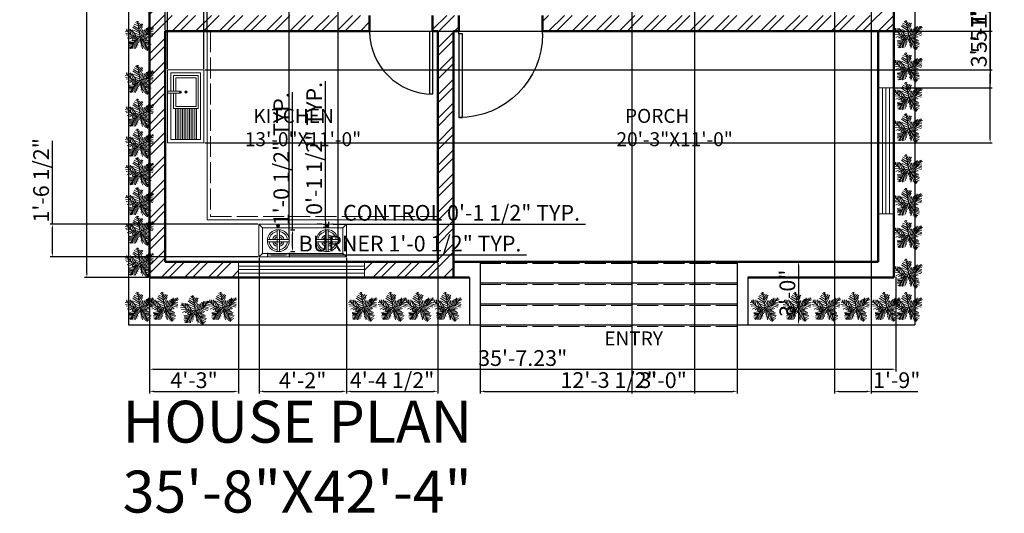
# Model space of a CAD drawing. Units: inches. Extents: x 176 to 806, y 915 to 1663.
# Tile 1 of 5: x 228 to 792, y 915 to 1198. Entities that reach past the tile are written whole.
import ezdxf

# ---------------------------------------------------------------- set-up
doc = ezdxf.new("R2010")
doc.units = ezdxf.units.IN
doc.linetypes.add('ACAD_ISO02W100', pattern=[15, 12, -3])
for name, color, linetype, lineweight in [('A-ANNO-DIMS', 2, 'Continuous', 18), ('A-ANNO-TEXT', 7, 'Continuous', 18), ('A-AREA-IDEN', 7, 'Continuous', 18), ('A-DOOR', 4, 'Continuous', 25), ('A-EQPM', 9, 'Continuous', 18), ('A-FLOR-CASE', 8, 'Continuous', 18), ('A-FLOR-CASE-HIDN', 8, 'ACAD_ISO02W100', 13), ('A-FLOR-FIXT', 9, 'Continuous', 18), ('A-FLOR-STRS', 7, 'Continuous', 25), ('A-FLOR-STRS-HIDN', 8, 'ACAD_ISO02W100', 13), ('A-WALL', 7, 'Continuous', 50), ('A-WALL-PATT', 252, 'Continuous', 13), ('C-PROP', 8, 'Continuous', 25), ('L-PLNT', 3, 'Continuous', 13)]:
    doc.layers.add(name, color=color, linetype=linetype, lineweight=lineweight)
doc.layers.add('A-GLAZ', color=244, linetype='Continuous', lineweight=18, true_color=0x991b1e)
doc.styles.get("Standard").update_dxf_attribs({"font": 'arial.ttf'})
doc.dimstyles.new('ISO-25', dxfattribs={"dimtxt": 9, "dimasz": 2.5, "dimexe": 1.25, "dimexo": 0.625, "dimtad": 1, "dimlunit": 3, "dimtxsty": 'Standard', "dimcen": 2.5, "dimadec": 0, "dimazin": 0, "dimtfac": 1, "dimtmove": 0, "dimatfit": 3, "dimfxl": 1, "dimarcsym": 0})

# ---------------------------------------------------------------- blocks, each defined once
blk = doc.blocks.new('*U2')
for p, q in [((-40, 0), (-40, 6)), ((0, 0), (0, 6))]:
    blk.add_line(p, q)
blk.add_lwpolyline([(0, 0), (0, -40), (-1.75, -40), (-1.75, 0)], close=True)
blk.add_arc((0, 0), 40, 180, 270)
blk = doc.blocks.new('*U8')
for p, q in [((-5.114, 28.097), (-24.676, 40.636)), ((-7.288, 39.707), (-21.778, 46.673)), ((-8.737, 47.138), (-17.069, 52.711)), ((-10.186, 53.64), (-13.084, 55.962)), ((0, 0), (-10.5, 57)), ((-9.099, 51.782), (-6.563, 55.962)), ((-7.65, 43.423), (-2.578, 49.46)), ((-5.839, 35.992), (4.667, 48.067)), ((-5.114, 27.632), (10.463, 46.673)), ((-2.941, 16.486), (8.652, 37.85)), ((-47.498, 19.737), (-55.83, 18.344)), ((-40.615, 13.7), (-55.105, 10.913)), ((-31.5, 4.5), (-52.5, 25.5)), ((-33.37, 6.269), (-52.207, 5.34)), ((-48.585, 21.131), (-49.309, 29.026)), ((-28.299, 3.483), (-47.86, -5.805)), ((-43.513, 28.561), (-42.427, 15.558)), ((-38.442, 26.239), (-34.819, 7.663)), ((-21.416, 3.018), (-38.079, -8.128)), ((-35.544, 28.097), (-24.314, 3.947)), ((0, 0), (-31.5, 4.5)), ((-14.533, 2.09), (-30.834, 25.31)), ((-15.982, 2.09), (-30.11, -9.521)), ((-3.665, 19.273), (-27.574, 35.527)), ((-24.314, 23.917), (-2.941, 13.7)), ((0, 0), (-22.5, -19.5)), ((-6.563, 1.161), (-21.416, -8.128)), ((-20.691, 13.7), (-1.129, 4.876)), ((-1.129, 6.734), (9.014, 26.704)), ((0, 0), (27, 9)), ((0, 0), (18, -22.5)), ((3.942, 1.625), (11.187, 24.381)), ((6.478, 1.625), (26.04, -8.592)), ((10.101, 3.483), (17.708, 26.239)), ((11.187, 3.483), (30.749, -5.805)), ((16.259, 5.805), (23.142, 31.348)), ((18.07, 5.805), (35.096, -3.483)), ((22.055, 7.198), (27.489, 32.277)), ((24.229, 7.663), (46.688, 1.625)), ((27, 9), (48, 36)), ((27.127, 9.056), (31.112, 35.992)), ((29.662, 12.307), (48.137, 6.269)), ((31.836, 30.883), (32.561, 16.486)), ((33.285, 16.486), (48.862, 10.913)), ((35.096, 32.741), (37.27, 22.524)), ((36.183, 19.737), (48.137, 17.88)), ((38.719, 34.134), (41.979, 28.561)), ((40.53, 25.775), (48.862, 24.846)), ((43.791, 29.954), (51.036, 30.883)), ((44.153, 36.456), (45.239, 32.741)), ((-17.431, -15.094), (-42.789, -18.809)), ((-28.299, -29.026), (-42.789, -31.348)), ((-24.314, -21.596), (-42.427, -22.06)), ((-30.834, -34.135), (-42.427, -35.528)), ((-26.849, -26.24), (-40.253, -25.775)), ((-22.5, -19.5), (-37.5, -45)), ((-15.257, -12.772), (-30.11, -12.772)), ((-29.023, -30.884), (-27.936, -43.887)), ((-25.038, -23.918), (-22.865, -45.281)), ((-20.691, -18.345), (-17.793, -44.352)), ((-6.563, -5.805), (-19.967, -9.985)), ((-17.069, -15.094), (-12.721, -40.172)), ((-13.446, -11.378), (-8.737, -32.741)), ((-9.461, -8.592), (-6.201, -23.453)), ((-4.752, -3.483), (-3.665, -14.629)), ((2.493, -3.019), (-1.491, -20.202)), ((1.769, -2.555), (24.229, -9.521)), ((5.029, -6.27), (2.131, -25.775)), ((9.014, -11.378), (3.58, -35.992)), ((14.085, -16.951), (6.478, -40.172)), ((7.565, -9.056), (32.198, -14.629)), ((18.07, -22.524), (8.289, -45.745)), ((12.274, -15.094), (36.907, -18.809)), ((20.244, -30.419), (15.897, -44.816)), ((16.259, -19.738), (36.183, -22.989)), ((18, -22.5), (27, -52.5)), ((18.433, -22.524), (40.53, -29.026)), ((19.157, -25.311), (38.719, -33.206)), ((21.331, -32.741), (39.081, -40.636)), ((-34.457, -39.708), (-40.978, -42.494)), ((-32.646, -36.921), (-31.921, -44.352)), ((22.78, -37.85), (19.519, -48.532)), ((22.78, -38.314), (34.372, -44.816)), ((24.591, -45.745), (23.142, -50.854)), ((24.591, -43.423), (30.749, -47.603)), ((26.764, -49.925), (28.213, -50.854))]:
    blk.add_line(p, q)
blk = doc.blocks.new('*D9')
at = {"layer": 'A-ANNO-DIMS', "color": 0, "lineweight": -2, "transparency": 16777216}
for p, q in [((302.7, 1049.58), (302.7, 996.47)), ((729.94, 1050.58), (729.94, 996.47)), ((305.2, 997.72), (727.44, 997.72))]:
    blk.add_line(p, q, dxfattribs=at)
at = {"layer": 'A-ANNO-DIMS', "color": 0, "transparency": 16777216}
for points in [[(305.2, 998.13), (305.2, 997.3), (302.7, 997.72)], [(727.44, 998.13), (727.44, 997.3), (729.94, 997.72)]]:
    blk.add_solid(points, dxfattribs=at)
at = {"layer": 'Defpoints', "color": 0, "transparency": 16777216}
for p in [(302.7, 1050.21), (729.94, 1051.2), (729.94, 997.72)]:
    blk.add_point(p, dxfattribs=at)
at = {"layer": 'A-ANNO-DIMS', "color": 0, "transparency": 16777216, "insert": (516.32, 1002.94), "char_height": 9, "attachment_point": 5}
blk.add_mtext('35\'-7.23"', dxfattribs=at)
blk = doc.blocks.new('*D10')
at = {"layer": 'A-ANNO-DIMS', "color": 0, "lineweight": -2, "transparency": 16777216}
for p, q in [((302.08, 1558.21), (265.58, 1558.21)), ((266.83, 1052.71), (266.83, 1555.71)), ((302.08, 1050.21), (265.58, 1050.21))]:
    blk.add_line(p, q, dxfattribs=at)
at = {"layer": 'A-ANNO-DIMS', "color": 0, "transparency": 16777216}
for points in [[(266.42, 1555.71), (267.25, 1555.71), (266.83, 1558.21)], [(266.42, 1052.71), (267.25, 1052.71), (266.83, 1050.21)]]:
    blk.add_solid(points, dxfattribs=at)
at = {"layer": 'Defpoints', "color": 0, "transparency": 16777216}
for p in [(266.83, 1558.21), (302.7, 1558.21), (302.7, 1050.21)]:
    blk.add_point(p, dxfattribs=at)
at = {"layer": 'A-ANNO-DIMS', "color": 0, "transparency": 16777216, "insert": (261.69, 1304.21), "char_height": 9, "attachment_point": 5, "rotation": 90}
blk.add_mtext('42\'-4"', dxfattribs=at)
blk = doc.blocks.new('WIN-GLAZING-72IN')
for p, q in [((0, 2), (72, 2)), ((0, 0), (72, 0)), ((0, -2), (72, -2))]:
    blk.add_line(p, q)
blk = doc.blocks.new('COOKTOP-BURNER')
for p, q in [((-0.6, 6.24), (-0.6, -6.24)), ((0.6, 6.24), (0.6, -6.24)), ((-6.24, 0.6), (6.24, 0.6)), ((-6.24, -0.6), (6.24, -0.6))]:
    blk.add_line(p, q)
blk.add_circle((0, 0), 6.27)
for radius, start, end in [(5.27, 96.5353, 173.4647), (3.27, 100.5674, 169.4326), (2.27, 105.3147, 164.6853), (5.27, 6.5353, 83.4647), (3.27, 10.5674, 79.4326), (2.27, 15.3147, 74.6853), (5.27, 186.5353, 263.4647), (3.27, 190.5674, 259.4326), (2.27, 195.3147, 254.6853), (5.27, 276.5353, 353.4647), (3.27, 280.5674, 349.4326), (2.27, 285.3147, 344.6853)]:
    blk.add_arc((0, 0), radius, start, end)
blk = doc.blocks.new('COOKTOP-CONTROL')
for p, q in [((-0.82, 0.2), (0.82, 0.2)), ((-0.82, -0.2), (0.82, -0.2))]:
    blk.add_line(p, q)
blk.add_circle((0, 0), 0.845)
for start, end in [(21.5247, 158.4753), (201.5247, 338.4753)]:
    blk.add_arc((0, 0), 0.545, start, end)
blk = doc.blocks.new('*D30')
at = {"layer": 'A-ANNO-DIMS', "color": 0, "lineweight": -2, "transparency": 16777216}
for p, q in [((370.15, 1064.42), (370.15, 1061.91)), ((372.65, 1063.16), (380.19, 1063.16)), ((382.69, 1064.42), (382.69, 1061.91)), ((382.69, 1063.16), (518.46, 1063.16))]:
    blk.add_line(p, q, dxfattribs=at)
at = {"layer": 'A-ANNO-DIMS', "color": 0, "transparency": 16777216}
for points in [[(372.65, 1063.58), (372.65, 1062.75), (370.15, 1063.16)], [(380.19, 1063.58), (380.19, 1062.75), (382.69, 1063.16)]]:
    blk.add_solid(points, dxfattribs=at)
at = {"layer": 'Defpoints', "color": 0, "transparency": 16777216}
for p in [(370.15, 1065.04), (382.69, 1065.04), (382.69, 1063.16)]:
    blk.add_point(p, dxfattribs=at)
at = {"layer": 'A-ANNO-DIMS', "color": 0, "transparency": 16777216, "insert": (451.83, 1068.44), "char_height": 9, "attachment_point": 5}
blk.add_mtext('BURNER 1\'-0 1/2" TYP.', dxfattribs=at)
blk = doc.blocks.new('*D31')
at = {"layer": 'A-ANNO-DIMS', "color": 0, "lineweight": -2, "transparency": 16777216}
for p, q in [((384.58, 1077.59), (384.58, 1156.32)), ((383.32, 1077.59), (385.83, 1077.59)), ((384.58, 1067.54), (384.58, 1075.09)), ((383.32, 1065.04), (385.83, 1065.04))]:
    blk.add_line(p, q, dxfattribs=at)
at = {"layer": 'A-ANNO-DIMS', "color": 0, "transparency": 16777216}
for points in [[(384.16, 1075.09), (384.99, 1075.09), (384.58, 1077.59)], [(384.16, 1067.54), (384.99, 1067.54), (384.58, 1065.04)]]:
    blk.add_solid(points, dxfattribs=at)
at = {"layer": 'Defpoints', "color": 0, "transparency": 16777216}
for p in [(382.69, 1077.59), (384.58, 1077.59), (382.69, 1065.04)]:
    blk.add_point(p, dxfattribs=at)
at = {"layer": 'A-ANNO-DIMS', "color": 0, "transparency": 16777216, "insert": (379.3, 1118.2), "char_height": 9, "attachment_point": 5, "rotation": 90}
blk.add_mtext('1\'-0 1/2" TYP.', dxfattribs=at)
blk = doc.blocks.new('*D32')
at = {"layer": 'A-ANNO-DIMS', "color": 0, "lineweight": -2, "transparency": 16777216}
for p, q in [((401.15, 1080.8), (398.65, 1080.8)), ((403.65, 1081.17), (403.65, 1082.05)), ((403.65, 1080.8), (405.34, 1080.8)), ((405.34, 1081.17), (405.34, 1082.05)), ((407.84, 1080.8), (552.28, 1080.8))]:
    blk.add_line(p, q, dxfattribs=at)
at = {"layer": 'A-ANNO-DIMS', "color": 0, "transparency": 16777216}
for points in [[(401.15, 1081.22), (401.15, 1080.38), (403.65, 1080.8)], [(407.84, 1081.22), (407.84, 1080.38), (405.34, 1080.8)]]:
    blk.add_solid(points, dxfattribs=at)
at = {"layer": 'Defpoints', "color": 0, "transparency": 16777216}
for p in [(403.65, 1080.55), (405.34, 1080.8), (405.34, 1080.55)]:
    blk.add_point(p, dxfattribs=at)
at = {"layer": 'A-ANNO-DIMS', "color": 0, "transparency": 16777216, "insert": (481.31, 1086.08), "char_height": 9, "attachment_point": 5}
blk.add_mtext('CONTROL 0\'-1 1/2" TYP.', dxfattribs=at)
blk = doc.blocks.new('*D33')
at = {"layer": 'A-ANNO-DIMS', "color": 0, "lineweight": -2, "transparency": 16777216}
for p, q in [((403.4, 1083.05), (403.4, 1162.63)), ((403.03, 1080.55), (402.15, 1080.55)), ((403.03, 1078.86), (402.15, 1078.86)), ((403.4, 1078.86), (403.4, 1080.55)), ((403.4, 1076.36), (403.4, 1073.86))]:
    blk.add_line(p, q, dxfattribs=at)
at = {"layer": 'A-ANNO-DIMS', "color": 0, "transparency": 16777216}
for points in [[(402.98, 1083.05), (403.81, 1083.05), (403.4, 1080.55)], [(402.98, 1076.36), (403.81, 1076.36), (403.4, 1078.86)]]:
    blk.add_solid(points, dxfattribs=at)
at = {"layer": 'Defpoints', "color": 0, "transparency": 16777216}
for p in [(403.4, 1080.55), (403.65, 1080.55), (403.65, 1078.86)]:
    blk.add_point(p, dxfattribs=at)
at = {"layer": 'A-ANNO-DIMS', "color": 0, "transparency": 16777216, "insert": (398.12, 1124.09), "char_height": 9, "attachment_point": 5, "rotation": 90}
blk.add_mtext('0\'-1 1/2" TYP.', dxfattribs=at)
blk = doc.blocks.new('*D47')
at = {"layer": 'A-ANNO-DIMS', "color": 0, "lineweight": -2, "transparency": 16777216}
for p, q in [((729.33, 1225.71), (785.1, 1225.71)), ((783.85, 1223.21), (783.85, 1161.23)), ((729.33, 1158.73), (785.1, 1158.73))]:
    blk.add_line(p, q, dxfattribs=at)
at = {"layer": 'A-ANNO-DIMS', "color": 0, "transparency": 16777216}
for points in [[(783.43, 1223.21), (784.27, 1223.21), (783.85, 1225.71)], [(783.43, 1161.23), (784.27, 1161.23), (783.85, 1158.73)]]:
    blk.add_solid(points, dxfattribs=at)
at = {"layer": 'Defpoints', "color": 0, "transparency": 16777216}
for p in [(728.7, 1225.71), (728.7, 1158.73), (783.85, 1158.73)]:
    blk.add_point(p, dxfattribs=at)
at = {"layer": 'A-ANNO-DIMS', "color": 0, "transparency": 16777216, "insert": (778.65, 1192.22), "char_height": 9, "attachment_point": 5, "rotation": 90}
blk.add_mtext('5\'-7"', dxfattribs=at)
blk = doc.blocks.new('*D49')
at = {"layer": 'A-ANNO-DIMS', "color": 0, "lineweight": -2, "transparency": 16777216}
for p, q in [((302.7, 1049.58), (302.7, 983.8)), ((353.7, 1049.58), (353.7, 983.8)), ((305.2, 985.05), (351.2, 985.05))]:
    blk.add_line(p, q, dxfattribs=at)
at = {"layer": 'A-ANNO-DIMS', "color": 0, "transparency": 16777216}
for points in [[(305.2, 985.47), (305.2, 984.64), (302.7, 985.05)], [(351.2, 985.47), (351.2, 984.64), (353.7, 985.05)]]:
    blk.add_solid(points, dxfattribs=at)
at = {"layer": 'Defpoints', "color": 0, "transparency": 16777216}
for p in [(302.7, 1050.21), (353.7, 1050.21), (353.7, 985.05)]:
    blk.add_point(p, dxfattribs=at)
at = {"layer": 'A-ANNO-DIMS', "color": 0, "transparency": 16777216, "insert": (328.2, 990.28), "char_height": 9, "attachment_point": 5}
blk.add_mtext('4\'-3"', dxfattribs=at)
blk = doc.blocks.new('*D51')
at = {"layer": 'A-ANNO-DIMS', "color": 0, "lineweight": -2, "transparency": 16777216}
for p, q in [((491.88, 1022.58), (491.88, 983.8)), ((639.17, 1022.58), (639.17, 983.8)), ((494.38, 985.05), (636.67, 985.05))]:
    blk.add_line(p, q, dxfattribs=at)
at = {"layer": 'A-ANNO-DIMS', "color": 0, "transparency": 16777216}
for points in [[(494.38, 985.47), (494.38, 984.64), (491.88, 985.05)], [(636.67, 985.47), (636.67, 984.64), (639.17, 985.05)]]:
    blk.add_solid(points, dxfattribs=at)
at = {"layer": 'Defpoints', "color": 0, "transparency": 16777216}
for p in [(491.88, 1023.21), (639.17, 1023.21), (639.17, 985.05)]:
    blk.add_point(p, dxfattribs=at)
at = {"layer": 'A-ANNO-DIMS', "color": 0, "transparency": 16777216, "insert": (565.52, 990.34), "char_height": 9, "attachment_point": 5}
blk.add_mtext('12\'-3 1/2"', dxfattribs=at)
blk = doc.blocks.new('*D55')
at = {"layer": 'A-ANNO-DIMS', "color": 0, "lineweight": -2, "transparency": 16777216}
for p, q in [((365.38, 1061.4), (365.38, 983.8)), ((415.42, 1061.4), (415.42, 983.8)), ((367.88, 985.05), (412.92, 985.05))]:
    blk.add_line(p, q, dxfattribs=at)
at = {"layer": 'A-ANNO-DIMS', "color": 0, "transparency": 16777216}
for points in [[(367.88, 985.47), (367.88, 984.64), (365.38, 985.05)], [(412.92, 985.47), (412.92, 984.64), (415.42, 985.05)]]:
    blk.add_solid(points, dxfattribs=at)
at = {"layer": 'Defpoints', "color": 0, "transparency": 16777216}
for p in [(365.38, 1062.02), (415.42, 1062.02), (415.42, 985.05)]:
    blk.add_point(p, dxfattribs=at)
at = {"layer": 'A-ANNO-DIMS', "color": 0, "transparency": 16777216, "insert": (390.4, 990.2), "char_height": 9, "attachment_point": 5}
blk.add_mtext('4\'-2"', dxfattribs=at)
blk = doc.blocks.new('*D56')
at = {"layer": 'A-ANNO-DIMS', "color": 0, "lineweight": -2, "transparency": 16777216}
for p, q in [((247.1, 1080.68), (247.1, 1128.48)), ((364.75, 1080.68), (245.85, 1080.68)), ((247.1, 1064.52), (247.1, 1078.18)), ((364.75, 1062.02), (245.85, 1062.02))]:
    blk.add_line(p, q, dxfattribs=at)
at = {"layer": 'A-ANNO-DIMS', "color": 0, "transparency": 16777216}
for points in [[(246.68, 1078.18), (247.52, 1078.18), (247.1, 1080.68)], [(246.68, 1064.52), (247.52, 1064.52), (247.1, 1062.02)]]:
    blk.add_solid(points, dxfattribs=at)
at = {"layer": 'Defpoints', "color": 0, "transparency": 16777216}
for p in [(247.1, 1080.68), (365.38, 1080.68), (365.38, 1062.02)]:
    blk.add_point(p, dxfattribs=at)
at = {"layer": 'A-ANNO-DIMS', "color": 0, "transparency": 16777216, "insert": (241.82, 1105.83), "char_height": 9, "attachment_point": 5, "rotation": 90}
blk.add_mtext('1\'-6 1/2"', dxfattribs=at)
blk = doc.blocks.new('*D57')
at = {"layer": 'A-ANNO-DIMS', "color": 0, "lineweight": -2, "transparency": 16777216}
for p, q in [((382.69, 1071.94), (382.69, 1645.51)), ((385.19, 1644.26), (408.14, 1644.26)), ((410.64, 1071.94), (410.64, 1645.51))]:
    blk.add_line(p, q, dxfattribs=at)
at = {"layer": 'A-ANNO-DIMS', "color": 0, "transparency": 16777216}
for points in [[(385.19, 1644.67), (385.19, 1643.84), (382.69, 1644.26)], [(408.14, 1644.67), (408.14, 1643.84), (410.64, 1644.26)]]:
    blk.add_solid(points, dxfattribs=at)
at = {"layer": 'Defpoints', "color": 0, "transparency": 16777216}
for p in [(410.64, 1644.26), (382.69, 1071.32), (410.64, 1071.32)]:
    blk.add_point(p, dxfattribs=at)
at = {"layer": 'A-ANNO-DIMS', "color": 0, "transparency": 16777216, "insert": (396.67, 1649.4), "char_height": 9, "attachment_point": 5}
blk.add_mtext('2\'-4"', dxfattribs=at)
blk = doc.blocks.new('*D60')
at = {"layer": 'A-ANNO-DIMS', "color": 0, "lineweight": -2, "transparency": 16777216}
for p, q in [((578.7, 1271.58), (578.7, 983.8)), ((614.7, 1271.58), (614.7, 983.8)), ((581.2, 985.05), (612.2, 985.05))]:
    blk.add_line(p, q, dxfattribs=at)
at = {"layer": 'A-ANNO-DIMS', "color": 0, "transparency": 16777216}
for points in [[(581.2, 985.47), (581.2, 984.64), (578.7, 985.05)], [(612.2, 985.47), (612.2, 984.64), (614.7, 985.05)]]:
    blk.add_solid(points, dxfattribs=at)
at = {"layer": 'Defpoints', "color": 0, "transparency": 16777216}
for p in [(578.7, 1272.21), (614.7, 1272.21), (614.7, 985.05)]:
    blk.add_point(p, dxfattribs=at)
at = {"layer": 'A-ANNO-DIMS', "color": 0, "transparency": 16777216, "insert": (596.7, 990.28), "char_height": 9, "attachment_point": 5}
blk.add_mtext('3\'-0"', dxfattribs=at)
blk = doc.blocks.new('*D61')
at = {"layer": 'A-ANNO-DIMS', "color": 0, "lineweight": -2, "transparency": 16777216}
for p, q in [((311.7, 1191.83), (311.7, 1645.51)), ((314.2, 1644.26), (333.2, 1644.26)), ((335.7, 1191.83), (335.7, 1645.51)), ((335.7, 1644.26), (363.53, 1644.26))]:
    blk.add_line(p, q, dxfattribs=at)
at = {"layer": 'A-ANNO-DIMS', "color": 0, "transparency": 16777216}
for points in [[(314.2, 1644.67), (314.2, 1643.84), (311.7, 1644.26)], [(333.2, 1644.67), (333.2, 1643.84), (335.7, 1644.26)]]:
    blk.add_solid(points, dxfattribs=at)
at = {"layer": 'Defpoints', "color": 0, "transparency": 16777216}
for p in [(335.7, 1644.26), (311.7, 1191.21), (335.7, 1191.21)]:
    blk.add_point(p, dxfattribs=at)
at = {"layer": 'A-ANNO-DIMS', "color": 0, "transparency": 16777216, "insert": (350.87, 1649.48), "char_height": 9, "attachment_point": 5}
blk.add_mtext('2\'-0"', dxfattribs=at)
blk = doc.blocks.new('*D62')
at = {"layer": 'A-ANNO-DIMS', "color": 0, "lineweight": -2, "transparency": 16777216}
for p, q in [((313.06, 1169.74), (313.06, 1645.51)), ((315.56, 1644.26), (331.24, 1644.26)), ((333.74, 1169.74), (333.74, 1645.51)), ((333.74, 1644.26), (381.54, 1644.26))]:
    blk.add_line(p, q, dxfattribs=at)
at = {"layer": 'A-ANNO-DIMS', "color": 0, "transparency": 16777216}
for points in [[(315.56, 1644.67), (315.56, 1643.84), (313.06, 1644.26)], [(331.24, 1644.67), (331.24, 1643.84), (333.74, 1644.26)]]:
    blk.add_solid(points, dxfattribs=at)
at = {"layer": 'Defpoints', "color": 0, "transparency": 16777216}
for p in [(333.74, 1644.26), (313.06, 1169.12), (333.74, 1169.12)]:
    blk.add_point(p, dxfattribs=at)
at = {"layer": 'A-ANNO-DIMS', "color": 0, "transparency": 16777216, "insert": (358.89, 1649.53), "char_height": 9, "attachment_point": 5}
blk.add_mtext('1\'-8 1/2"', dxfattribs=at)
blk = doc.blocks.new('*D63')
at = {"layer": 'A-ANNO-DIMS', "color": 0, "lineweight": -2, "transparency": 16777216}
for p, q in [((783.85, 1169.12), (783.85, 1217.75)), ((334.37, 1169.12), (785.1, 1169.12)), ((783.85, 1129.89), (783.85, 1166.62)), ((334.37, 1127.39), (785.1, 1127.39))]:
    blk.add_line(p, q, dxfattribs=at)
at = {"layer": 'A-ANNO-DIMS', "color": 0, "transparency": 16777216}
for points in [[(783.43, 1166.62), (784.27, 1166.62), (783.85, 1169.12)], [(783.43, 1129.89), (784.27, 1129.89), (783.85, 1127.39)]]:
    blk.add_solid(points, dxfattribs=at)
at = {"layer": 'Defpoints', "color": 0, "transparency": 16777216}
for p in [(333.74, 1169.12), (783.85, 1169.12), (333.74, 1127.39)]:
    blk.add_point(p, dxfattribs=at)
at = {"layer": 'A-ANNO-DIMS', "color": 0, "transparency": 16777216, "insert": (778.57, 1194.68), "char_height": 9, "attachment_point": 5, "rotation": 90}
blk.add_mtext('3\'-5 1/2"', dxfattribs=at)
blk = doc.blocks.new('*D67')
at = {"layer": 'A-ANNO-DIMS', "color": 0, "lineweight": -2, "transparency": 16777216}
for p, q in [((783.85, 1191.21), (783.85, 1225.03)), ((336.33, 1191.21), (785.1, 1191.21)), ((783.85, 1171.62), (783.85, 1188.71)), ((334.37, 1169.12), (785.1, 1169.12))]:
    blk.add_line(p, q, dxfattribs=at)
at = {"layer": 'A-ANNO-DIMS', "color": 0, "transparency": 16777216}
for points in [[(783.43, 1188.71), (784.27, 1188.71), (783.85, 1191.21)], [(783.43, 1171.62), (784.27, 1171.62), (783.85, 1169.12)]]:
    blk.add_solid(points, dxfattribs=at)
at = {"layer": 'Defpoints', "color": 0, "transparency": 16777216}
for p in [(335.7, 1191.21), (783.85, 1191.21), (333.74, 1169.12)]:
    blk.add_point(p, dxfattribs=at)
at = {"layer": 'A-ANNO-DIMS', "color": 0, "transparency": 16777216, "insert": (778.63, 1209.37), "char_height": 9, "attachment_point": 5, "rotation": 90}
blk.add_mtext('1\'-10"', dxfattribs=at)
blk = doc.blocks.new('*D68')
at = {"layer": 'A-ANNO-DIMS', "color": 0, "lineweight": -2, "transparency": 16777216}
for p, q in [((415.42, 1061.4), (415.42, 983.8)), ((467.7, 1058.58), (467.7, 983.8)), ((417.92, 985.05), (465.2, 985.05))]:
    blk.add_line(p, q, dxfattribs=at)
at = {"layer": 'A-ANNO-DIMS', "color": 0, "transparency": 16777216}
for points in [[(417.92, 985.47), (417.92, 984.64), (415.42, 985.05)], [(465.2, 985.47), (465.2, 984.64), (467.7, 985.05)]]:
    blk.add_solid(points, dxfattribs=at)
at = {"layer": 'Defpoints', "color": 0, "transparency": 16777216}
for p in [(415.42, 1062.02), (467.7, 1059.21), (467.7, 985.05)]:
    blk.add_point(p, dxfattribs=at)
at = {"layer": 'A-ANNO-DIMS', "color": 0, "transparency": 16777216, "insert": (441.56, 990.33), "char_height": 9, "attachment_point": 5}
blk.add_mtext('4\'-4 1/2"', dxfattribs=at)
blk = doc.blocks.new('*D70')
at = {"layer": 'A-ANNO-DIMS', "color": 0, "lineweight": -2, "transparency": 16777216}
for p, q in [((694.73, 1263.58), (694.73, 983.8)), ((715.73, 1263.58), (715.73, 983.8)), ((697.23, 985.05), (713.23, 985.05)), ((715.73, 985.05), (742.56, 985.05))]:
    blk.add_line(p, q, dxfattribs=at)
at = {"layer": 'A-ANNO-DIMS', "color": 0, "transparency": 16777216}
for points in [[(697.23, 985.47), (697.23, 984.64), (694.73, 985.05)], [(713.23, 985.47), (713.23, 984.64), (715.73, 985.05)]]:
    blk.add_solid(points, dxfattribs=at)
at = {"layer": 'Defpoints', "color": 0, "transparency": 16777216}
for p in [(694.73, 1264.21), (715.73, 1264.21), (715.73, 985.05)]:
    blk.add_point(p, dxfattribs=at)
at = {"layer": 'A-ANNO-DIMS', "color": 0, "transparency": 16777216, "insert": (730.4, 990.27), "char_height": 9, "attachment_point": 5}
blk.add_mtext('1\'-9"', dxfattribs=at)
blk = doc.blocks.new('*D73')
at = {"layer": 'A-ANNO-DIMS', "color": 0, "lineweight": -2, "transparency": 16777216}
for p, q in [((639.79, 1059.21), (675.47, 1059.21)), ((674.22, 1056.71), (674.22, 1025.71)), ((639.79, 1023.21), (675.47, 1023.21))]:
    blk.add_line(p, q, dxfattribs=at)
at = {"layer": 'A-ANNO-DIMS', "color": 0, "transparency": 16777216}
for points in [[(673.8, 1056.71), (674.64, 1056.71), (674.22, 1059.21)], [(673.8, 1025.71), (674.64, 1025.71), (674.22, 1023.21)]]:
    blk.add_solid(points, dxfattribs=at)
at = {"layer": 'Defpoints', "color": 0, "transparency": 16777216}
for p in [(639.17, 1059.21), (639.17, 1023.21), (674.22, 1023.21)]:
    blk.add_point(p, dxfattribs=at)
at = {"layer": 'A-ANNO-DIMS', "color": 0, "transparency": 16777216, "insert": (669, 1041.21), "char_height": 9, "attachment_point": 5, "rotation": 90}
blk.add_mtext('3\'-0"', dxfattribs=at)

msp = doc.modelspace()

# ---------------------------------------------------------------- hatches: boundary and pattern name
at = {"layer": 'A-WALL-PATT'}
h = msp.add_hatch(dxfattribs=at)
h.set_pattern_fill('ANSI32', color=256)
h.paths.add_polyline_path([(302.704, 1050.206), (353.704, 1050.206), (353.704, 1059.206), (311.704, 1059.206), (311.704, 1191.206), (428.704, 1191.206), (428.704, 1200.206), (311.704, 1200.206), (311.704, 1357.206), (473.704, 1357.206), (473.704, 1363.206), (408.704, 1363.206), (408.704, 1366.206), (402.704, 1366.206), (402.704, 1363.206), (311.704, 1363.206), (311.704, 1376.706), (302.704, 1376.706)])
h.paths.add_polyline_path([(311.704, 1447.206), (302.704, 1447.206), (302.704, 1397.706), (311.704, 1397.706), (311.704, 1411.206), (402.704, 1411.206), (402.704, 1396.206), (408.704, 1396.206), (408.704, 1411.206), (473.704, 1411.206), (473.704, 1420.206), (467.704, 1420.206), (467.704, 1417.206), (311.704, 1417.206)])
h.paths.add_polyline_path([(467.704, 1059.206), (425.704, 1059.206), (425.704, 1050.206), (476.704, 1050.206), (476.704, 1191.206), (479.704, 1191.206), (479.704, 1200.206), (464.704, 1200.206), (464.704, 1191.206), (467.704, 1191.206)])
h.paths.add_polyline_path([(719.704, 1278.206), (614.704, 1278.206), (614.704, 1272.206), (654.704, 1272.206), (654.704, 1250.311), (660.704, 1250.311), (660.704, 1272.206), (719.704, 1272.206), (719.704, 1246.706), (728.704, 1246.706), (728.704, 1307.669), (719.704, 1307.669)])
h.paths.add_polyline_path([(728.704, 1447.206), (719.704, 1447.206), (719.704, 1417.206), (563.704, 1417.206), (563.704, 1420.206), (557.704, 1420.206), (557.704, 1411.206), (569.704, 1411.206), (569.704, 1272.206), (578.704, 1272.206), (578.704, 1278.206), (575.704, 1278.206), (575.704, 1411.206), (719.704, 1411.206), (719.704, 1379.669), (728.704, 1379.669)])
h.paths.add_polyline_path([(677.704, 1558.206), (677.704, 1549.206), (719.704, 1549.206), (719.704, 1519.206), (728.704, 1519.206), (728.704, 1558.206)])
h.paths.add_polyline_path([(526.204, 1558.206), (526.204, 1549.206), (557.704, 1549.206), (557.704, 1481.206), (554.704, 1481.206), (554.704, 1475.206), (557.704, 1475.206), (557.704, 1456.206), (563.704, 1456.206), (563.704, 1549.206), (605.704, 1549.206), (605.704, 1558.206)])
h.paths.add_polyline_path([(425.704, 1558.206), (425.704, 1549.206), (467.704, 1549.206), (467.704, 1456.206), (473.704, 1456.206), (473.704, 1475.206), (524.704, 1475.206), (524.704, 1481.206), (473.704, 1481.206), (473.704, 1549.206), (505.204, 1549.206), (505.204, 1558.206)])
h.paths.add_polyline_path([(311.704, 1549.206), (353.704, 1549.206), (353.704, 1558.206), (302.704, 1558.206), (302.704, 1519.206), (311.704, 1519.206)])
h = msp.add_hatch(dxfattribs=at)
h.set_pattern_fill('ANSI32', color=256)
h.paths.add_polyline_path([(719.704, 1200.206), (660.704, 1200.206), (660.704, 1220.311), (656.204, 1220.311), (654.704, 1220.311), (654.704, 1200.206), (527.704, 1200.206), (527.704, 1191.206), (728.704, 1191.206), (728.704, 1225.706), (719.704, 1225.706)])

# ---------------------------------------------------------------- linework, layer by layer
at = {"layer": 'A-EQPM'}
for p, q in [((367.375, 1078.683), (365.375, 1080.683)), ((413.42, 1078.683), (415.42, 1080.683)), ((367.375, 1064.021), (365.375, 1062.021)), ((413.42, 1064.021), (415.42, 1062.021))]:
    msp.add_line(p, q, dxfattribs=at)
for points in [[(365.375, 1080.683), (415.42, 1080.683), (415.42, 1062.021), (365.375, 1062.021)], [(367.375, 1078.683), (413.42, 1078.683), (413.42, 1064.021), (367.375, 1064.021)]]:
    msp.add_lwpolyline(points, close=True, dxfattribs=at)
at = {"layer": 'A-FLOR-CASE'}
for p, q in [((335.704, 1191.206), (335.704, 1083.206)), ((335.704, 1083.206), (467.704, 1083.206))]:
    msp.add_line(p, q, dxfattribs=at)
at = {"layer": 'A-FLOR-CASE-HIDN'}
for p, q in [((337.704, 1191.206), (337.704, 1085.206)), ((337.704, 1085.206), (467.704, 1085.206))]:
    msp.add_line(p, q, dxfattribs=at)
at = {"layer": 'A-FLOR-FIXT'}
for p, q in [((320.424, 1156.919), (313.064, 1156.919)), ((320.424, 1155.719), (313.064, 1155.719)), ((322.914, 1156.319), (324.233, 1156.319)), ((323.108, 1155.853), (324.039, 1156.786)), ((324.027, 1155.841), (323.124, 1156.801)), ((323.573, 1156.978), (323.573, 1155.66)), ((317.573, 1146.856), (317.573, 1129.186)), ((318.573, 1146.856), (318.573, 1129.186)), ((319.573, 1146.856), (319.573, 1129.186)), ((320.573, 1146.856), (320.573, 1129.186)), ((321.573, 1146.856), (321.573, 1129.186)), ((322.573, 1146.856), (322.573, 1129.186)), ((323.573, 1146.856), (323.573, 1129.186)), ((324.573, 1146.856), (324.573, 1129.186)), ((325.573, 1146.856), (325.573, 1129.186)), ((326.573, 1146.856), (326.573, 1129.186)), ((327.573, 1146.856), (327.573, 1129.186)), ((328.573, 1146.856), (328.573, 1129.186)), ((329.573, 1146.856), (329.573, 1129.186))]:
    msp.add_line(p, q, dxfattribs=at)
msp.add_lwpolyline([(313.064, 1169.115), (333.742, 1169.115), (333.742, 1127.386), (313.064, 1127.386)], close=True, dxfattribs=at)
for points in [[(314.864, 1156.919), (314.864, 1167.315), (331.942, 1167.315), (331.942, 1129.186), (314.864, 1129.186), (314.864, 1155.719)], [(316.534, 1156.919), (316.534, 1165.782), (330.613, 1165.782), (330.613, 1146.856), (316.534, 1146.856), (316.534, 1155.719)], [(317.734, 1156.919), (317.734, 1164.582), (329.413, 1164.582), (329.413, 1148.056), (317.734, 1148.056), (317.734, 1155.719)]]:
    msp.add_lwpolyline(points, dxfattribs=at)
for centre, radius in [((320.424, 1156.319), 0.6), ((320.424, 1156.319), 0.316), ((323.573, 1156.319), 0.659), ((323.573, 1156.319), 0.459)]:
    msp.add_circle(centre, radius, dxfattribs=at)
at = {"layer": 'A-FLOR-STRS'}
for p, q in [((491.88, 1059.206), (491.88, 1023.206)), ((639.17, 1059.206), (639.17, 1023.206)), ((485.88, 1050.206), (485.88, 1023.206)), ((645.17, 1050.206), (645.17, 1023.206)), ((491.88, 1047.206), (639.17, 1047.206)), ((491.88, 1035.206), (639.17, 1035.206))]:
    msp.add_line(p, q, dxfattribs=at)
at = {"layer": 'A-FLOR-STRS-HIDN'}
for p, q in [((491.88, 1058.206), (639.17, 1058.206)), ((491.88, 1046.206), (639.17, 1046.206)), ((491.88, 1034.206), (639.17, 1034.206)), ((491.88, 1022.206), (639.17, 1022.206))]:
    msp.add_line(p, q, dxfattribs=at)
at = {"layer": 'A-GLAZ'}
for points in [[(728.704, 1158.726), (728.704, 1086.726), (719.704, 1086.726), (719.704, 1158.726)], [(353.704, 1059.206), (425.704, 1059.206), (425.704, 1050.206), (353.704, 1050.206)]]:
    msp.add_lwpolyline(points, close=True, dxfattribs=at)
at = {"layer": 'A-WALL'}
for p, q in [((302.704, 1558.206), (302.704, 1050.206)), ((728.704, 1558.206), (728.704, 1050.206)), ((428.704, 1191.206), (428.704, 1200.206)), ((464.704, 1191.206), (464.704, 1200.206)), ((479.704, 1191.206), (479.704, 1200.206)), ((527.704, 1191.206), (527.704, 1200.206)), ((311.704, 1191.206), (428.704, 1191.206)), ((311.704, 1191.206), (311.704, 1059.206)), ((464.704, 1191.206), (467.704, 1191.206)), ((467.704, 1191.206), (467.704, 1059.206)), ((476.704, 1191.206), (476.704, 1050.206)), ((476.704, 1191.206), (479.704, 1191.206)), ((527.704, 1191.206), (728.704, 1191.206)), ((719.704, 1191.206), (719.704, 1059.206)), ((311.704, 1059.206), (467.704, 1059.206)), ((476.704, 1059.206), (719.704, 1059.206)), ((302.704, 1050.206), (485.88, 1050.206)), ((645.17, 1050.206), (728.704, 1050.206))]:
    msp.add_line(p, q, dxfattribs=at)
at = {"layer": 'C-PROP'}
for p, q in [((290.704, 1570.206), (290.704, 1023.206)), ((740.704, 1570.206), (740.704, 1023.206)), ((290.704, 1023.206), (740.704, 1023.206))]:
    msp.add_line(p, q, dxfattribs=at)

# ---------------------------------------------------------------- block references
at = {"layer": 'A-DOOR'}
for p, xscale, yscale, zscale in [((464.704, 1191.206), 0.9, 0.9, 0.9), ((479.704, 1189.706), -1.2, 1.2, 1.2)]:
    msp.add_blockref('*U2', p, dxfattribs=dict(at, xscale=xscale, yscale=yscale, zscale=zscale))
at = {"layer": 'A-EQPM'}
for name, p in [('COOKTOP-BURNER', (376.423, 1071.316)), ('COOKTOP-CONTROL', (376.299, 1079.702)), ('COOKTOP-BURNER', (404.372, 1071.316)), ('COOKTOP-CONTROL', (404.496, 1079.702))]:
    msp.add_blockref(name, p, dxfattribs=at)
at = {"layer": 'A-GLAZ'}
for p, rotation in [((724.204, 1086.726), 90), ((425.704, 1054.706), 180)]:
    msp.add_blockref('WIN-GLAZING-72IN', p, dxfattribs=dict(at, rotation=rotation))
at = {"layer": 'L-PLNT', "xscale": 0.1538165911341002, "yscale": 0.1538165911341002, "zscale": 0.1538165911341002}
for p in [(297.354, 1188.097), (737.299, 1188.544), (737.299, 1170.126), (297.354, 1162.995), (737.299, 1153.213), (297.354, 1143.629), (737.299, 1135.337), (297.354, 1126.467), (297.354, 1110.138), (737.299, 1111.83), (297.354, 1092.962), (737.299, 1092.623), (297.354, 1076.634), (737.299, 1074.167), (297.354, 1058.407), (737.299, 1052.094), (297.354, 1033.018), (311.469, 1033.018), (328.999, 1031.161), (344.88, 1033.018), (425.211, 1033.018), (442.142, 1033.018), (457.686, 1033.018), (473.588, 1033.018), (655.199, 1033.018), (673.854, 1033.018), (690.5, 1033.018), (707.147, 1033.018), (724.671, 1033.018), (737.299, 1033.018)]:
    msp.add_blockref('*U8', p, dxfattribs=at)

# ---------------------------------------------------------------- texts
at = {"layer": 'A-ANNO-TEXT', "attachment_point": 1}
for s, width, insert, char_height in [('ENTRY', 38.13266, (563.007, 1019.366), 8), ('HOUSE PLAN\\P35\'-8"X42\'-4"', 217.54927, (287.371, 979.684), 24)]:
    msp.add_mtext_dynamic_manual_height_columns(s, width=width, gutter_width=12.5, heights=[0], dxfattribs=dict(at, insert=insert, char_height=char_height))
at = {"layer": 'A-AREA-IDEN', "char_height": 8, "attachment_point": 1}
for s, insert in [('  KITCHEN 13\'-0"X11\'-0"', (357.277, 1146.709)), ('  PORCH 20\'-3"X11\'-0"', (570.004, 1146.709))]:
    msp.add_mtext_dynamic_manual_height_columns(s, width=64.1724, gutter_width=12.5, heights=[0], dxfattribs=dict(at, insert=insert))

# ---------------------------------------------------------------- dimensions: what is measured, and where the dimension line sits
at = {"layer": 'A-ANNO-DIMS'}
for base, p1, p2, override, picture, middle in [((333.742, 1644.256), (313.064, 1169.115), (333.742, 1169.115), {"dimdec": 1, "dimlfac": 1, "dimrnd": 0, "dimzin": 1, "dimdsep": 46, "dimlunit": 4, "dimfrac": 2}, '*D62', (358.892, 1649.535)), ((335.704, 1644.256), (311.704, 1191.206), (335.704, 1191.206), {"dimdec": 1, "dimlfac": 1, "dimrnd": 0, "dimzin": 1, "dimdsep": 46, "dimlunit": 4, "dimfrac": 2}, '*D61', (350.868, 1649.477)), ((410.644, 1644.256), (382.695, 1071.316), (410.644, 1071.316), {"dimdec": 1, "dimlfac": 1, "dimrnd": 0, "dimzin": 1, "dimdsep": 46, "dimlunit": 4, "dimfrac": 2}, '*D57', (396.669, 1649.4)), ((614.704, 985.054), (578.704, 1272.206), (614.704, 1272.206), {"dimdec": 1, "dimlfac": 1, "dimrnd": 0, "dimzin": 1, "dimdsep": 46, "dimlunit": 4, "dimfrac": 2}, '*D60', (596.704, 990.277)), ((715.734, 985.054), (694.734, 1264.206), (715.734, 1264.206), {"dimdec": 1, "dimlfac": 1, "dimrnd": 0, "dimzin": 1, "dimdsep": 46, "dimlunit": 4, "dimfrac": 2}, '*D70', (730.398, 990.274)), ((415.42, 985.054), (365.375, 1062.021), (415.42, 1062.021), {"dimdec": 1, "dimlfac": 1, "dimrnd": 0, "dimzin": 1, "dimdsep": 46, "dimlunit": 4, "dimfrac": 2}, '*D55', (390.397, 990.197)), ((467.704, 985.054), (415.42, 1062.021), (467.704, 1059.206), {"dimdec": 1, "dimlfac": 1, "dimrnd": 0, "dimzin": 1, "dimdsep": 46, "dimlunit": 4, "dimfrac": 2}, '*D68', (441.562, 990.332)), ((729.937, 997.716), (302.704, 1050.206), (729.937, 1051.201), {"dimclrd": 0, "dimclre": 0, "dimclrt": 0}, '*D9', (516.321, 1002.939)), ((353.704, 985.054), (302.704, 1050.206), (353.704, 1050.206), {"dimdec": 1, "dimlfac": 1, "dimrnd": 0, "dimzin": 1, "dimdsep": 46, "dimlunit": 4, "dimfrac": 2}, '*D49', (328.204, 990.277)), ((639.17, 985.054), (491.88, 1023.206), (639.17, 1023.206), {"dimdec": 1, "dimlfac": 1, "dimrnd": 0, "dimzin": 1, "dimdsep": 46, "dimlunit": 4, "dimfrac": 2}, '*D51', (565.525, 990.335))]:
    dim = msp.add_linear_dim(base=base, p1=p1, p2=p2, dimstyle='ISO-25', override=override, dxfattribs=at)
    dim.commit()
    dim.dimension.update_dxf_attribs({"geometry": picture, "text_midpoint": middle})
for base, p1, p2, angle, override, picture, middle in [((266.833, 1558.206), (302.704, 1050.206), (302.704, 1558.206), 90, {"dimclrd": 0, "dimclre": 0, "dimclrt": 0}, '*D10', (261.689, 1304.206)), ((783.849, 1191.206), (333.742, 1169.115), (335.704, 1191.206), 90, {"dimdec": 1, "dimlfac": 1, "dimrnd": 0, "dimzin": 1, "dimdsep": 46, "dimlunit": 4, "dimfrac": 2}, '*D67', (778.629, 1209.366)), ((783.849, 1158.726), (728.704, 1225.706), (728.704, 1158.726), 90, {"dimdec": 1, "dimlfac": 1, "dimrnd": 0, "dimzin": 1, "dimdsep": 46, "dimlunit": 4, "dimfrac": 2}, '*D47', (778.647, 1192.216)), ((783.849, 1169.115), (333.742, 1127.386), (333.742, 1169.115), 90, {"dimdec": 1, "dimlfac": 1, "dimrnd": 0, "dimzin": 1, "dimdsep": 46, "dimlunit": 4, "dimfrac": 2}, '*D63', (778.568, 1194.685)), ((247.1, 1080.683), (365.375, 1062.021), (365.375, 1080.683), 90, {"dimdec": 1, "dimlfac": 1, "dimrnd": 0, "dimzin": 1, "dimdsep": 46, "dimlunit": 4, "dimfrac": 2}, '*D56', (241.821, 1105.832)), ((674.22, 1023.206), (639.17, 1059.206), (639.17, 1023.206), 270, {"dimdec": 1, "dimlfac": 1, "dimrnd": 0, "dimzin": 1, "dimdsep": 46, "dimlunit": 4, "dimfrac": 2}, '*D73', (668.997, 1041.206))]:
    dim = msp.add_linear_dim(base=base, p1=p1, p2=p2, angle=angle, dimstyle='ISO-25', override=override, dxfattribs=at)
    dim.commit()
    dim.dimension.update_dxf_attribs({"geometry": picture, "text_midpoint": middle})
for base, p1, p2, picture, middle in [((403.397, 1080.547), (403.651, 1078.857), (403.651, 1080.547), '*D33', (398.119, 1124.088)), ((384.576, 1077.587), (382.695, 1065.044), (382.695, 1077.587), '*D31', (379.298, 1118.204))]:
    dim = msp.add_linear_dim(base=base, p1=p1, p2=p2, angle=90, text='<> TYP.', dimstyle='ISO-25', override={"dimdec": 1, "dimlfac": 1, "dimrnd": 0, "dimzin": 1, "dimdsep": 46, "dimlunit": 4, "dimfrac": 2}, dxfattribs=at)
    dim.commit()
    dim.dimension.update_dxf_attribs({"geometry": picture, "text_midpoint": middle})
for base, p1, p2, text, picture, middle in [((405.341, 1080.801), (403.651, 1080.547), (405.341, 1080.547), 'CONTROL <> TYP.', '*D32', (481.312, 1086.082)), ((382.695, 1063.163), (370.151, 1065.044), (382.695, 1065.044), 'BURNER <> TYP.', '*D30', (451.828, 1068.441))]:
    dim = msp.add_linear_dim(base=base, p1=p1, p2=p2, text=text, dimstyle='ISO-25', override={"dimdec": 1, "dimlfac": 1, "dimrnd": 0, "dimzin": 1, "dimdsep": 46, "dimlunit": 4, "dimfrac": 2}, dxfattribs=at)
    dim.commit()
    dim.dimension.update_dxf_attribs({"geometry": picture, "text_midpoint": middle})

doc.saveas('drawing.dxf')
